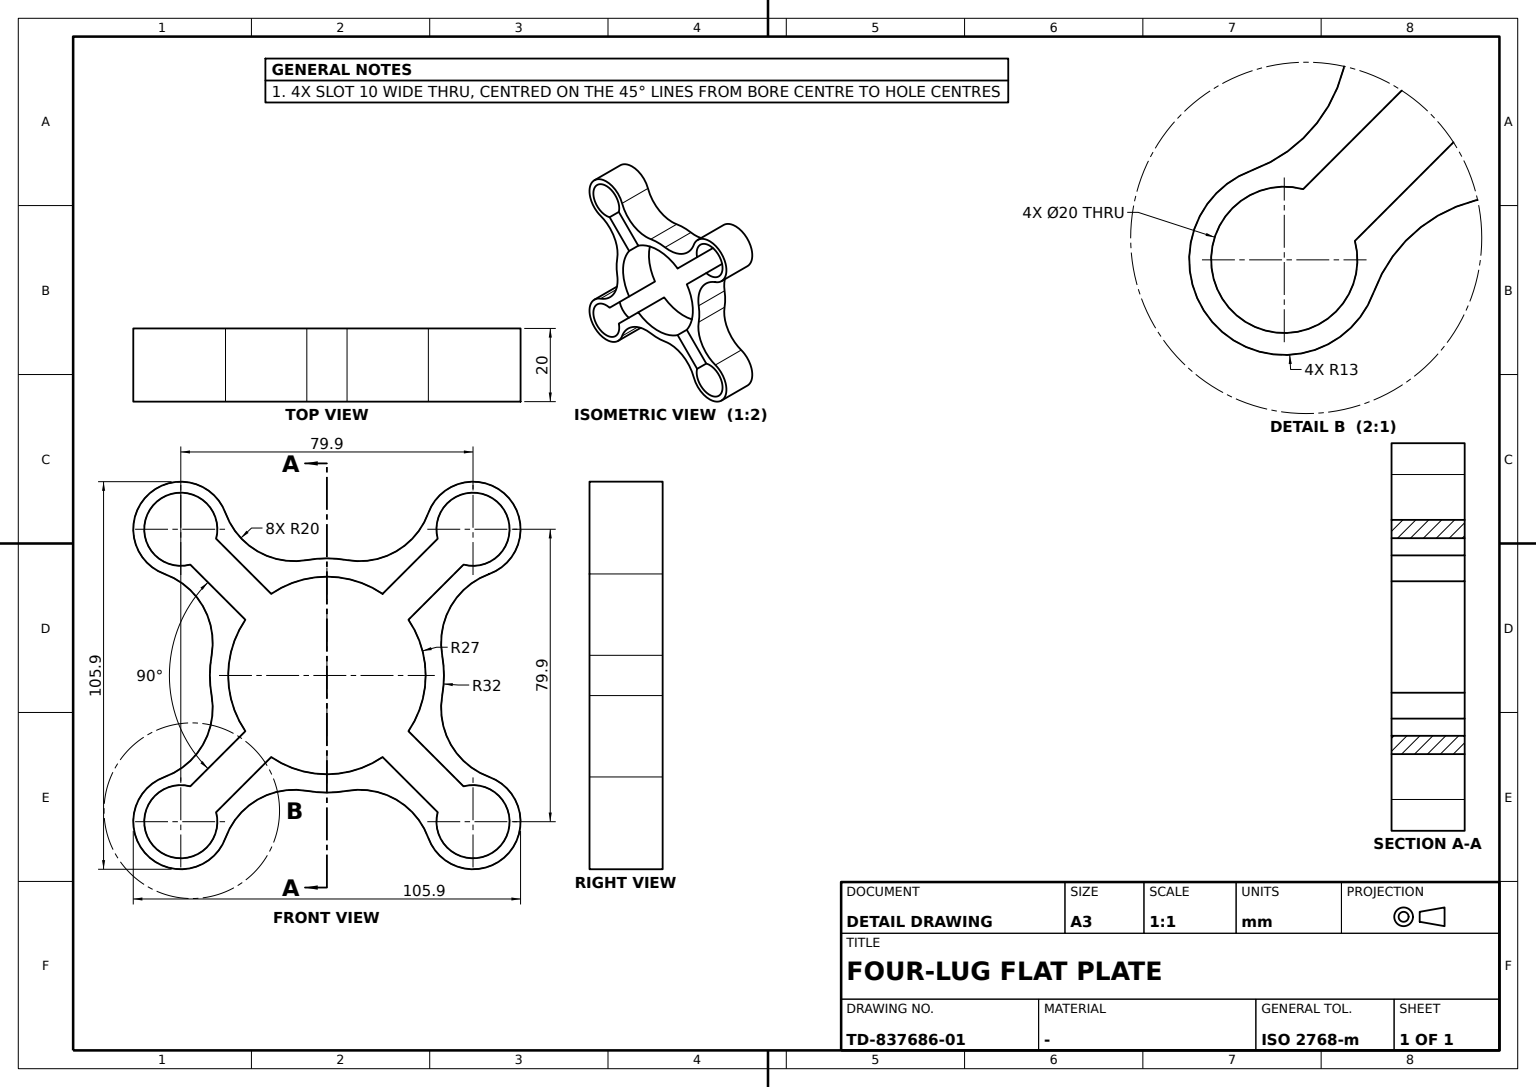
CATIA V5 part; units mm, degrees
sketch "Sketch1" plane through (0, 0, 0) normal (1, 0, 0) x (0, 1, 0)
  arc A0 (5.4999, 31.5238) -> (-5.4999, 31.5238) centre (0, 0) ccw construction
  arc A1 (15.2261, 22.2972) -> (-15.2261, 22.2972) centre (0, 0) ccw
  line L0 (0, 0) -> (64.1138, 64.1138) construction
  line L1 (-65.8556, 0) -> (97.9114, 0) construction
  point P0 (-65.8556, 0)
  circle A2 centre (0, 0) radius 56.5 construction
  line L2 (15.2261, 22.2972) -> (30.2923, 37.3633)
  line L3 (22.2972, 15.2261) -> (37.3633, 30.2923)
  arc A3 (37.3633, 30.2923) -> (30.2923, 37.3633) centre (39.9515, 39.9515) ccw
  point P1 (39.9515, 39.9515)
  point P2 (-30.2923, 37.3633)
  point P3 (-15.2261, 22.2972)
  line L4 (-15.2261, 22.2972) -> (-30.2923, 37.3633)
  point P4 (-37.3633, 30.2923)
  point P5 (-22.2972, 15.2261)
  line L5 (-22.2972, 15.2261) -> (-37.3633, 30.2923)
  arc A4 (-30.2923, 37.3633) -> (-37.3633, 30.2923) centre (-39.9515, 39.9515) ccw
  line L6 (-22.2972, -15.2261) -> (-37.3633, -30.2923)
  line L7 (-15.2261, -22.2972) -> (-30.2923, -37.3633)
  arc A5 (-37.3633, -30.2923) -> (-30.2923, -37.3633) centre (-39.9515, -39.9515) ccw
  arc A6 (-31.5238, 5.4999) -> (-31.5238, -5.4999) centre (0, 0) ccw construction
  arc A7 (-22.2972, 15.2261) -> (-22.2972, -15.2261) centre (0, 0) ccw
  arc A8 (-5.4999, -31.5238) -> (5.4999, -31.5238) centre (0, 0) ccw construction
  arc A9 (-15.2261, -22.2972) -> (15.2261, -22.2972) centre (0, 0) ccw
  arc A10 (31.5238, -5.4999) -> (31.5238, 5.4999) centre (0, 0) ccw construction
  arc A11 (22.2972, -15.2261) -> (22.2972, 15.2261) centre (0, 0) ccw
  arc A12 (44.3931, 27.7338) -> (27.7338, 44.3931) centre (39.9515, 39.9515) ccw
  point P6 (-51.7618, 36.0858)
  arc A13 (-27.7338, 44.3931) -> (-44.3931, 27.7338) centre (-39.9515, 39.9515) ccw
  arc A14 (-44.3931, -27.7338) -> (-27.7338, -44.3931) centre (-39.9515, -39.9515) ccw
  arc A15 (5.4999, 31.5238) -> (27.7338, 44.3931) centre (8.9373, 51.2262) ccw
  point P7 (28.7678, 48.6278)
  point P8 (5.4999, 31.5238)
  point P9 (31.5238, 5.4999)
  arc A16 (31.5238, 5.4999) -> (44.3931, 27.7338) centre (51.2262, 8.9373) cw
  point P10 (-44.3931, 27.7338)
  point P11 (-31.5238, 5.4999)
  arc A17 (-31.5238, 5.4999) -> (-44.3931, 27.7338) centre (-51.2262, 8.9373) ccw
  point P12 (-27.7338, 44.3931)
  point P13 (-5.4999, 31.5238)
  arc A18 (-5.4999, 31.5238) -> (-27.7338, 44.3931) centre (-8.9373, 51.2262) cw
  arc A19 (-5.4999, -31.5238) -> (-27.7338, -44.3931) centre (-8.9373, -51.2262) ccw
  arc A20 (-31.5238, -5.4999) -> (-44.3931, -27.7338) centre (-51.2262, -8.9373) cw
  point P14 (31.5238, -5.4999)
  line L8 (0, 0) -> (-57.9366, 57.9366) construction
  point P15 (56.9218, -49.8508)
  arc A21 (5.4999, 31.5238) -> (-5.4999, 31.5238) centre (0, 0) ccw
  point P16 (-32, 0)
  arc A22 (-31.5238, 5.4999) -> (-31.5238, -5.4999) centre (0, 0) ccw
  arc A23 (-5.4999, -31.5238) -> (5.4999, -31.5238) centre (0, 0) ccw
  line L9 (0, 0) -> (71.3685, -71.3685) construction
  point P17 (30.2923, -37.3633)
  point P18 (15.2261, -22.2972)
  line L10 (15.2261, -22.2972) -> (30.2923, -37.3633)
  point P19 (27.7338, -44.3931)
  point P20 (5.4999, -31.5238)
  arc A24 (5.4999, -31.5238) -> (27.7338, -44.3931) centre (8.9373, -51.2262) cw
  point P21 (37.3633, -30.2923)
  point P22 (22.2972, -15.2261)
  line L11 (22.2972, -15.2261) -> (37.3633, -30.2923)
  arc A25 (37.3633, -30.2923) -> (30.2923, -37.3633) centre (39.9515, -39.9515) cw
  point P23 (44.3931, -27.7338)
  arc A26 (44.3931, -27.7338) -> (27.7338, -44.3931) centre (39.9515, -39.9515) cw
  point P24 (31.5238, -5.4999)
  arc A27 (31.5238, -5.4999) -> (44.3931, -27.7338) centre (51.2262, -8.9373) ccw
  arc A28 (31.5238, -5.4999) -> (31.5238, 5.4999) centre (0, 0) ccw
  dimension "radius A0" = 32
  dimension "radius A1" = 27
  dimension "angle L1 L0" = 45
  dimension "radius A2" = 56.5
  dimension "distance L3 L2" = 10
  dimension "distance L3 L0" = 5
  dimension "radius A3" = 10
  dimension "radius A12" = 13
  dimension "radius A15" = 20
  dimension "angle L8 L1" = 45
  dimension "distance L8 L5" = 5
  dimension "distance L5 L4" = 10
  dimension "radius A4" = 10
  dimension "radius A18" = 20
  dimension "length L5" = 21.3067
  dimension "length L4" = 21.3067
  dimension "radius A13" = 13
  dimension "angle L9 L1" = 45
  constraint coincidence P0 x-axis
  constraint coincidence P1 A2
  constraint coincidence P1 L0
  constraint coincidence A0 A6
  constraint coincidence A1 A7
  constraint coincidence A6 A8
  constraint coincidence A7 A9
  constraint coincidence A8 A10
  constraint coincidence A9 A11
  constraint coincidence A2 P7
  constraint coincidence P15 L4
  constraint coincidence A21 P16
  constraint coincidence P16 A6
  constraint coincidence P16 L1
  constraint coincidence A21 A22
  constraint coincidence A22 A23
  constraint coincidence A23 A28
  constraint coincidence P14 P24
  constraint horizontal L1 x-axis
  constraint tangency A15 A0
  constraint tangency A15 A12
  constraint symmetry P8 P9 L0
  constraint symmetry A15 A16 L0
  constraint symmetry P4 P17 L0
  constraint symmetry P5 P18 L0
  constraint symmetry L5 L10 L0
  constraint symmetry P10 P19 L0
  constraint symmetry P11 P20 L0
  constraint symmetry A17 A24 L0
  constraint symmetry P2 P21 L0
  constraint symmetry P3 P22 L0
  constraint symmetry L4 L11 L0
  constraint symmetry A4 A25 L0
  constraint symmetry P12 P23 L0
  constraint symmetry A13 A26 L0
  constraint symmetry P13 P24 L0
  constraint symmetry A18 A27 L0
extrude "Pad1" add sketch "Sketch1" along normal mid plane 20
